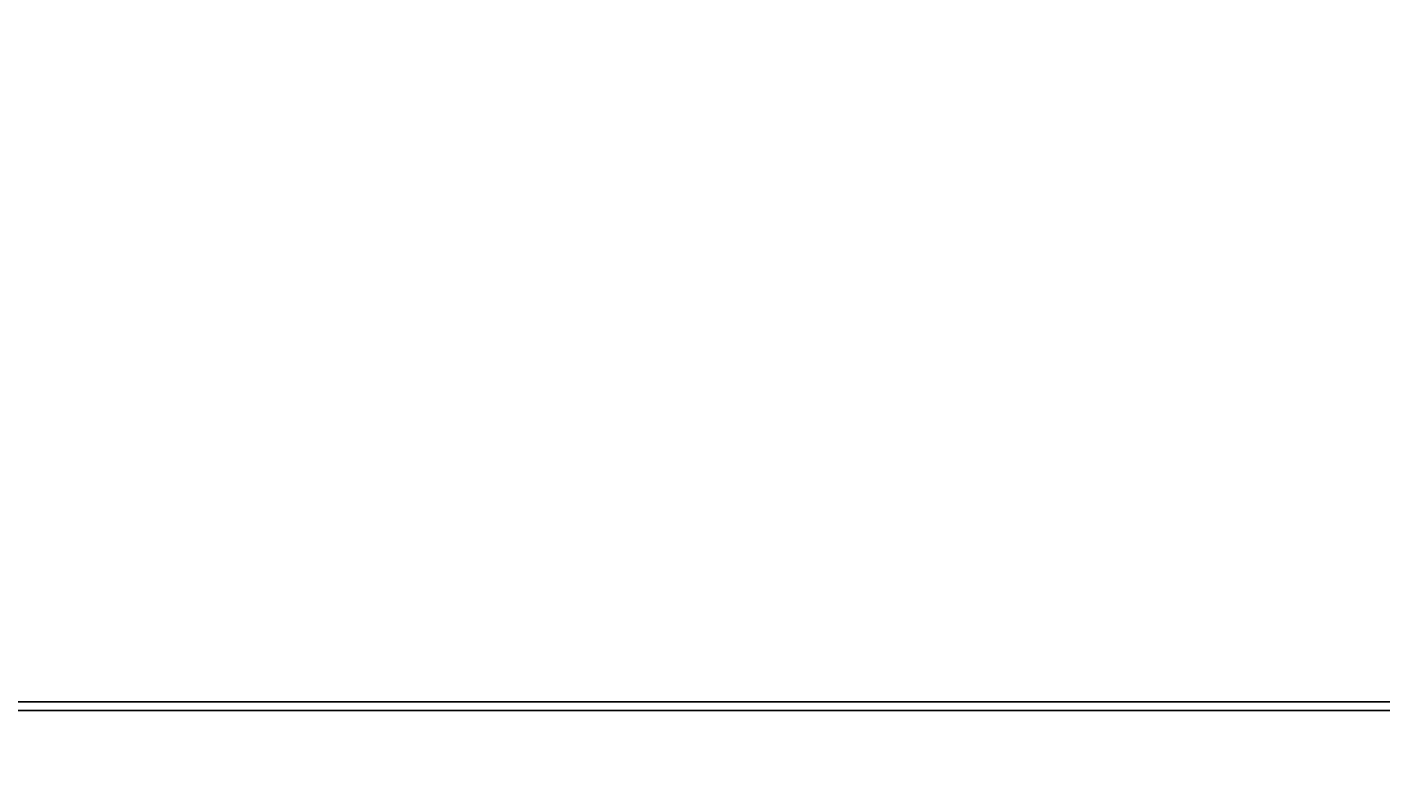
# Model space of a CAD drawing. Units: inches. Extents: x 35362 to 73946, y 43607 to 67532.
# Tile 71 of 134: x 48464 to 49302, y 49269 to 49738. Entities that reach past the tile are written whole.
import ezdxf

# ---------------------------------------------------------------- set-up
doc = ezdxf.new("R2010")
doc.units = ezdxf.units.IN
doc.header["$MEASUREMENT"] = 0
doc.layers.add('A-ANNO-DIMS', color=2, linetype='Continuous', lineweight=18)
doc.styles.get("Standard").update_dxf_attribs({"font": 'arial.ttf'})
doc.dimstyles.get("Standard").update_dxf_attribs({"dimtxt": 0.18, "dimasz": 0.18, "dimexe": 0.18, "dimexo": 0.0625, "dimgap": 0.09, "dimtad": 0, "dimtih": 1, "dimtoh": 1, "dimdec": 4, "dimzin": 0, "dimdsep": 46, "dimtxsty": 'Standard', "dimcen": 0.09, "dimadec": 0, "dimazin": 0, "dimtfac": 1, "dimtdec": 4, "dimtofl": 0, "dimtmove": 0, "dimatfit": 3, "dimfxl": 1, "dimtolj": 1, "dimtzin": 0, "dimarcsym": 0})

# ---------------------------------------------------------------- blocks, each defined once
blk = doc.blocks.new('*D11')
at = {"layer": 'A-ANNO-DIMS', "color": 0, "lineweight": -2, "transparency": 16777216}
for p, q in [((47978.66, 56028.77), (47978.66, 43606.68)), ((53109.76, 56028.77), (53109.76, 43606.68)), ((47978.84, 43606.86), (50543.87, 43606.86)), ((53109.58, 43606.86), (50544.55, 43606.86))]:
    blk.add_line(p, q, dxfattribs=at)
at = {"layer": 'A-ANNO-DIMS', "color": 0, "transparency": 16777216}
for points in [[(47978.84, 43606.89), (47978.84, 43606.83), (47978.66, 43606.86)], [(53109.58, 43606.89), (53109.58, 43606.83), (53109.76, 43606.86)]]:
    blk.add_solid(points, dxfattribs=at)
at = {"layer": 'Defpoints', "color": 0, "transparency": 16777216}
for p in [(47978.66, 56028.84), (53109.76, 56028.84), (53109.76, 43606.86)]:
    blk.add_point(p, dxfattribs=at)
at = {"layer": 'A-ANNO-DIMS', "color": 0, "transparency": 16777216, "insert": (50544.21, 43606.86), "char_height": 0.18, "attachment_point": 5}
blk.add_mtext('\\A1;5131', dxfattribs=at)
blk = doc.blocks.new('*D13')
at = {"layer": 'A-ANNO-DIMS', "color": 0, "lineweight": -2, "transparency": 16777216}
for p, q in [((48373.49, 51694.02), (48373.49, 43606.68)), ((51029.04, 51694.02), (51029.04, 43606.68)), ((48373.67, 43606.86), (49700.8, 43606.86)), ((51028.86, 43606.86), (49701.73, 43606.86))]:
    blk.add_line(p, q, dxfattribs=at)
at = {"layer": 'A-ANNO-DIMS', "color": 0, "transparency": 16777216}
for points in [[(48373.67, 43606.89), (48373.67, 43606.83), (48373.49, 43606.86)], [(51028.86, 43606.89), (51028.86, 43606.83), (51029.04, 43606.86)]]:
    blk.add_solid(points, dxfattribs=at)
at = {"layer": 'Defpoints', "color": 0, "transparency": 16777216}
for p in [(48373.49, 51694.09), (51029.04, 51694.09), (51029.04, 43606.86)]:
    blk.add_point(p, dxfattribs=at)
at = {"layer": 'A-ANNO-DIMS', "color": 0, "transparency": 16777216, "insert": (49701.27, 43606.86), "char_height": 0.18, "attachment_point": 5}
blk.add_mtext('\\A1;2655.6', dxfattribs=at)
blk = doc.blocks.new('*D40')
at = {"layer": 'A-ANNO-DIMS', "color": 0, "lineweight": -2, "transparency": 16777216}
for p, q in [((56873.54, 53351.53), (35361.77, 53351.53)), ((35361.95, 53351.35), (35361.95, 51333.28)), ((35361.95, 49314.85), (35361.95, 51332.92)), ((51806.45, 49314.67), (35361.77, 49314.67))]:
    blk.add_line(p, q, dxfattribs=at)
at = {"layer": 'A-ANNO-DIMS', "color": 0, "transparency": 16777216}
for points in [[(35361.92, 53351.35), (35361.98, 53351.35), (35361.95, 53351.53)], [(35361.92, 49314.85), (35361.98, 49314.85), (35361.95, 49314.67)]]:
    blk.add_solid(points, dxfattribs=at)
at = {"layer": 'Defpoints', "color": 0, "transparency": 16777216}
for p in [(35361.95, 53351.53), (56873.6, 53351.53), (51806.52, 49314.67)]:
    blk.add_point(p, dxfattribs=at)
at = {"layer": 'A-ANNO-DIMS', "color": 0, "transparency": 16777216, "insert": (35361.95, 51333.1), "char_height": 0.18, "attachment_point": 5}
blk.add_mtext('\\A1;4036.9', dxfattribs=at)
blk = doc.blocks.new('*D67')
at = {"layer": 'A-ANNO-DIMS', "color": 0, "lineweight": -2, "transparency": 16777216}
for p, q in [((56873.54, 53351.53), (35361.77, 53351.53)), ((35361.95, 53351.35), (35361.95, 49400.89)), ((35361.95, 45450.07), (35361.95, 49400.53)), ((53793.58, 45449.89), (35361.77, 45449.89))]:
    blk.add_line(p, q, dxfattribs=at)
at = {"layer": 'A-ANNO-DIMS', "color": 0, "transparency": 16777216}
for points in [[(35361.92, 53351.35), (35361.98, 53351.35), (35361.95, 53351.53)], [(35361.92, 45450.07), (35361.98, 45450.07), (35361.95, 45449.89)]]:
    blk.add_solid(points, dxfattribs=at)
at = {"layer": 'Defpoints', "color": 0, "transparency": 16777216}
for p in [(35361.95, 53351.53), (56873.6, 53351.53), (53793.64, 45449.89)]:
    blk.add_point(p, dxfattribs=at)
at = {"layer": 'A-ANNO-DIMS', "color": 0, "transparency": 16777216, "insert": (35361.95, 49400.71), "char_height": 0.18, "attachment_point": 5}
blk.add_mtext('\\A1;7901.6', dxfattribs=at)
blk = doc.blocks.new('*D86')
at = {"layer": 'A-ANNO-DIMS', "color": 0, "lineweight": -2, "transparency": 16777216}
for p, q in [((51285.53, 49320.08), (35361.77, 49320.08)), ((35361.95, 49319.9), (35361.95, 49120.26)), ((35361.95, 48920.26), (35361.95, 49119.9)), ((51285.53, 48920.08), (35361.77, 48920.08))]:
    blk.add_line(p, q, dxfattribs=at)
at = {"layer": 'A-ANNO-DIMS', "color": 0, "transparency": 16777216}
for points in [[(35361.92, 49319.9), (35361.98, 49319.9), (35361.95, 49320.08)], [(35361.92, 48920.26), (35361.98, 48920.26), (35361.95, 48920.08)]]:
    blk.add_solid(points, dxfattribs=at)
at = {"layer": 'Defpoints', "color": 0, "transparency": 16777216}
for p in [(35361.95, 49320.08), (51285.59, 49320.08), (51285.59, 48920.08)]:
    blk.add_point(p, dxfattribs=at)
at = {"layer": 'A-ANNO-DIMS', "color": 0, "transparency": 16777216, "insert": (35361.95, 49120.08), "char_height": 0.18, "attachment_point": 5}
blk.add_mtext('\\A1;400.0', dxfattribs=at)

msp = doc.modelspace()

# ---------------------------------------------------------------- dimensions: what is measured, and where the dimension line sits
at = {"layer": 'A-ANNO-DIMS'}
for base, p1, p2, override, picture, middle in [((53109.76, 43606.859), (47978.665, 56028.836), (53109.76, 56028.836), {"dimdec": 0, "dimlfac": 1, "dimrnd": 0, "dimzin": 0, "dimdsep": 46, "dimlunit": 2}, '*D11', (50544.212, 43606.859)), ((51029.043, 43606.859), (48373.492, 51694.087), (51029.043, 51694.087), {"dimdec": 1, "dimlfac": 1, "dimrnd": 0, "dimzin": 0, "dimdsep": 46, "dimlunit": 2}, '*D13', (49701.267, 43606.859))]:
    dim = msp.add_linear_dim(base=base, p1=p1, p2=p2, dimstyle='Standard', override=override, dxfattribs=at)
    dim.commit()
    dim.dimension.update_dxf_attribs({"geometry": picture, "text_midpoint": middle})
for base, p1, p2, picture, middle in [((35361.949, 53351.529), (51806.517, 49314.669), (56873.602, 53351.529), '*D40', (35361.949, 51333.099)), ((35361.949, 53351.529), (53793.638, 45449.894), (56873.602, 53351.529), '*D67', (35361.949, 49400.712)), ((35361.949, 49320.079), (51285.595, 48920.079), (51285.595, 49320.079), '*D86', (35361.949, 49120.079))]:
    dim = msp.add_linear_dim(base=base, p1=p1, p2=p2, angle=90, dimstyle='Standard', override={"dimdec": 1, "dimlfac": 1, "dimrnd": 0, "dimzin": 0, "dimdsep": 46, "dimlunit": 2}, dxfattribs=at)
    dim.commit()
    dim.dimension.update_dxf_attribs({"geometry": picture, "text_midpoint": middle})

doc.saveas('drawing.dxf')
